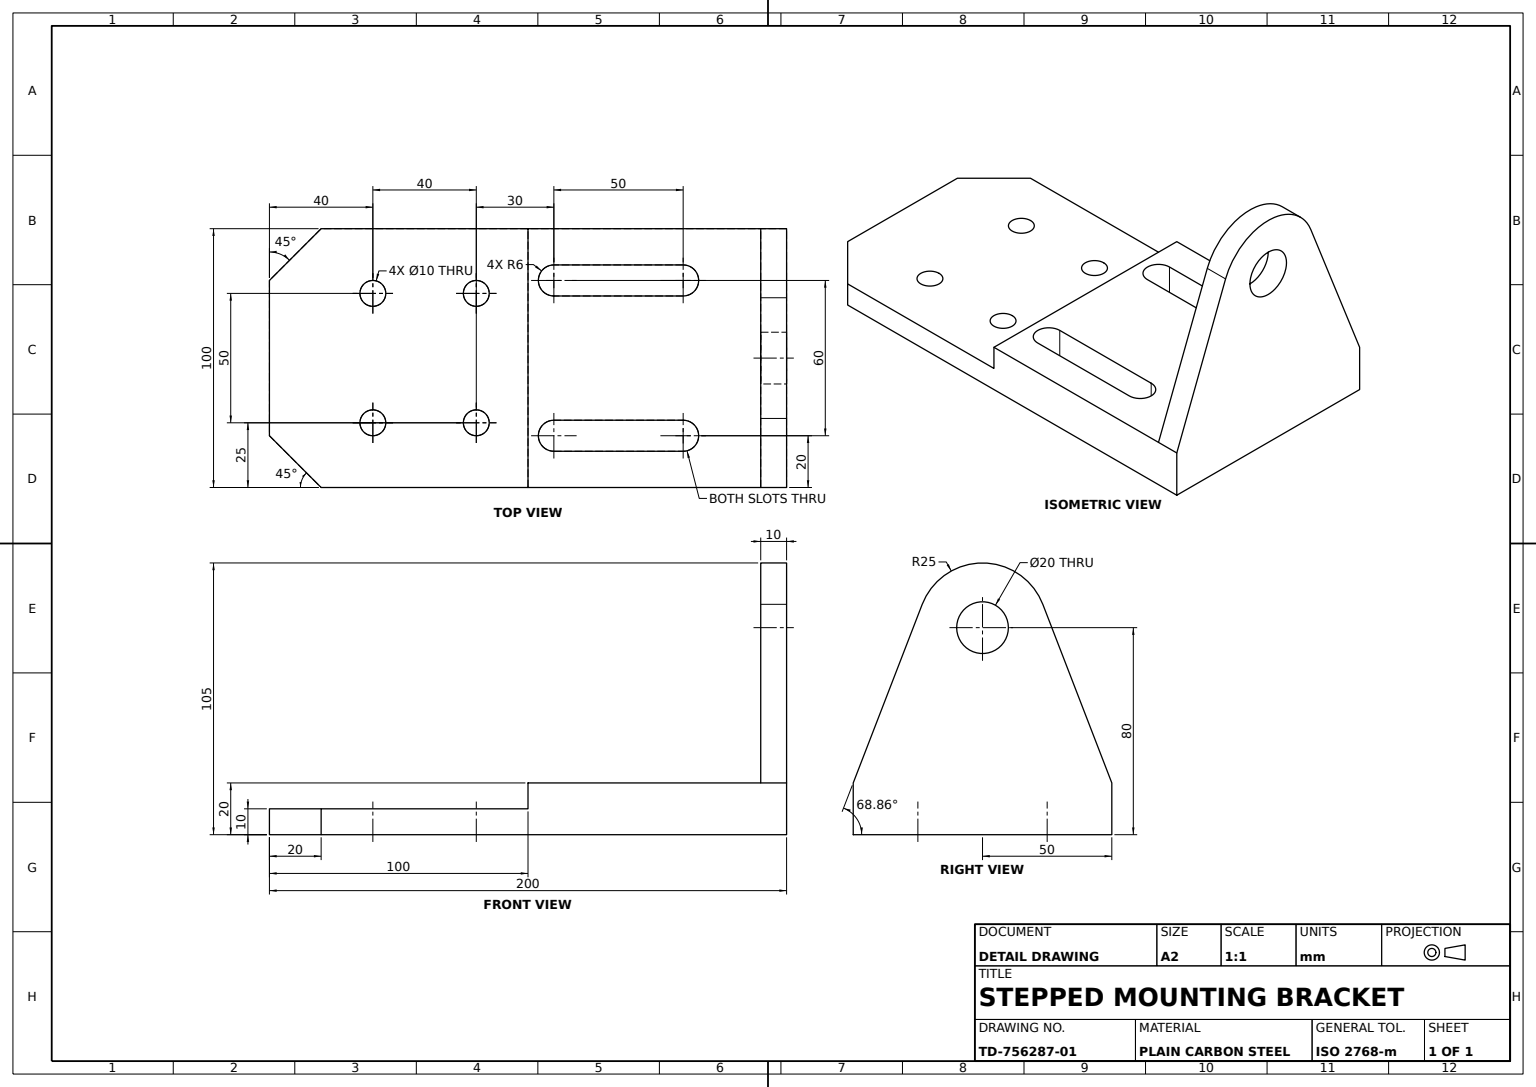
SolidWorks part; units mm, degrees
material "Plain Carbon Steel"
ref_plane "Front Plane" through (0, 0, 0) normal (0, 0, 1) x (1, 0, 0)
ref_plane "Top Plane" through (0, 0, 0) normal (0, 1, 0) x (1, 0, 0)
ref_plane "Right Plane" through (0, 0, 0) normal (1, 0, 0) x (0, 0, -1)
sketch "Base Plate Sketch" plane through (0, 0, 0) normal (0, 0, 1) x (1, 0, 0)
  line L0 (0, 0) -> (100, 0)
  line L1 (100, 0) -> (100, 20)
  line L2 (100, 20) -> (0, 20)
  line L3 (0, 20) -> (0, 0)
  dimension "D1" = 100
  dimension "D2" = 20
extrude "Base Plate" add sketch "Base Plate Sketch" along normal blind 100
ref_plane "Plane1" through (0, 0, 0) normal (0, 1, 0) x (1, 0, 0)
sketch "Mounting Flange Sketch" plane through (0, 0, 0) normal (0, 1, 0) x (1, 0, 0)
  line L2 (0, 0) -> (-100, 0)
  line L3 (-100, 0) -> (-100, -100)
  line L4 (-100, -100) -> (0, -100)
  line L5 (0, -100) -> (0, 0)
extrude "Mounting Flange" add sketch "Mounting Flange Sketch" along normal blind 10
chamfer "Flange Corner Chamfer 20mm" distance 20 angle 45 2 edges at (-100, 5, 100) (-100, 5, 0)
ref_plane "Plane2" through (100, 0, 0) normal (1, 0, 0) x (0, 0, -1)
sketch "Lug Profile Sketch" plane through (100, 0, 0) normal (1, 0, 0) x (0, 0, -1)
  line L0 (-50, 20) -> (-50, 80) construction
  line L1 (-100, 20) -> (0, 20) construction
  line L2 (-100, 20) -> (-73.318, 89.015)
  line L3 (0, 20) -> (-26.682, 89.015)
  line L4 (-100, 0) -> (-100, 20) construction
  line L5 (-100, 20) -> (0, 20)
  arc A0 (-26.682, 89.015) -> (-73.318, 89.015) centre (-50, 80) ccw
  circle A1 centre (-50, 80) radius 10
  dimension "D1" = 50
  dimension "D2" = 20
  dimension "D3" = 23.318
extrude "Upright Lug" add sketch "Lug Profile Sketch" against normal blind 10
sketch "Adjustment Slots Sketch" plane through (0, 20, 0) normal (0, 1, 0) x (1, 0, 0)
  line L0 (10, -20) -> (60, -20) construction
  line L1 (10, -14) -> (60, -14)
  line L2 (10, -26) -> (60, -26)
  line L3 (90, 0) -> (90, -26.682) construction
  line L4 (90, 0) -> (0, 0) construction
  line L5 (60, -80) -> (10, -80) construction
  line L6 (60, -86) -> (10, -86)
  line L7 (60, -74) -> (10, -74)
  line L8 (90, -100) -> (90, 0) construction
  line L9 (90, -100) -> (0, -100) construction
  arc A0 (10, -14) -> (10, -26) centre (10, -20) ccw
  arc A1 (60, -26) -> (60, -14) centre (60, -20) ccw
  arc A2 (60, -86) -> (60, -74) centre (60, -80) ccw
  arc A3 (10, -74) -> (10, -86) centre (10, -80) ccw
  point P2 (35, -20)
  point P13 (35, -80)
  dimension "D3" = 6
  dimension "D6" = 6
  dimension "D1" = 50
  dimension "D2" = 30
  dimension "D4" = 20
  dimension "D5" = 50
  dimension "D7" = 30
  dimension "D8" = 20
extrude "Adjustment Slots 2x" cut sketch "Adjustment Slots Sketch" against normal through all
sketch "Mounting Holes Sketch" plane through (0, 10, 0) normal (0, 1, 0) x (1, 0, 0)
  line L0 (-100, -50) -> (-100, -25) construction
  line L1 (-100, -20) -> (-100, -80) construction
  line L2 (-100, -25) -> (0, -25) construction
  line L3 (0, -100) -> (0, 0) construction
  line L4 (-100, -50) -> (-100, -75) construction
  line L5 (-100, -75) -> (0, -75) construction
  line L6 (0, -100) -> (0, 0) construction
  line L7 (-80, -100) -> (0, -100) construction
  circle A0 centre (-20, -25) radius 5
  circle A1 centre (-60, -25) radius 5
  circle A2 centre (-20, -75) radius 5
  circle A3 centre (-60, -75) radius 5
  dimension "D1" = 10
  dimension "D3" = 40
  dimension "D4" = 25
  dimension "D2" = 20
extrude "Flange Mounting Holes" cut sketch "Mounting Holes Sketch" against normal blind 10
